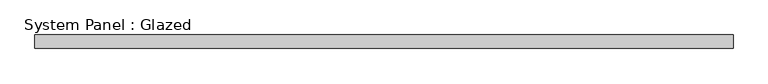
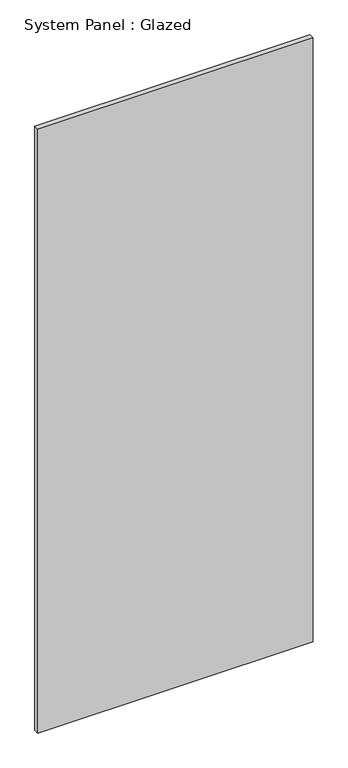
"""IFC4 building model written with IfcOpenShell, lengths in millimetres: plate geometry, System Panel : Glazed."""

from ifc_helpers import new_model, si_unit, origin, origin_with_axes, place, context, project, spatial, polyline, outline, extrude, source, transform, mapped, element, save


def system_panel_glazed_349e9711(model_context):
    return source(origin(), model_context, "Body", "SweptSolid", [
        extrude(outline(polyline([(657.225, 19.05), (-657.225, 19.05), (-657.225, 44.45), (657.225, 44.45), (657.225, 19.05)])), origin_with_axes(), (0.0, 0.0, 1.0), 3048.0),
    ])


if __name__ == "__main__":
    model = new_model("IFC4")
    model_context = context("Model", 3, world=origin())
    ifc_project = project(units=[si_unit("LENGTHUNIT", "METRE", prefix="MILLI")], contexts=[model_context])
    site = spatial("IfcSite", under=ifc_project)
    building = spatial("IfcBuilding", under=site)
    placement = place(None, origin())
    system_panel_glazed_shape = system_panel_glazed_349e9711(model_context)
    element("IfcPlate", 1, ObjectType="System Panel : Glazed", at=placement, inside=building, context=model_context, shape_type="MappedRepresentation", body=[
        mapped(system_panel_glazed_shape, transform((0.0, 0.0, 0.0), x_axis=(1.0, 0.0, 0.0), y_axis=(0.0, 1.0, 0.0), z_axis=(0.0, 0.0, 1.0))),
    ])
    save(model, "model.ifc")

# Revit data of these elements
# Type "System Panel : Glazed"
#   Construction Type Id = "GSP4R"
#   Analytic Construction = "1/8 in Pilkington single glazing"
#   Visual Light Transmittance = 0.9
#   Solar Heat Gain Coefficient = 0.86
#   Heat Transfer Coefficient (U) = 1.18115 BTU/(h·ft²·°F)
#   Define Thermal Properties by = 1
# Element 1 (IfcPlate, "System Panel : Glazed")
#   Materials on its faces: "Glass"
# Materials
#   "Glass": class "Glass", colour RGB 0 128 192, transparency 0.75, Description = "Soda Lime Glass", Cost = 0
